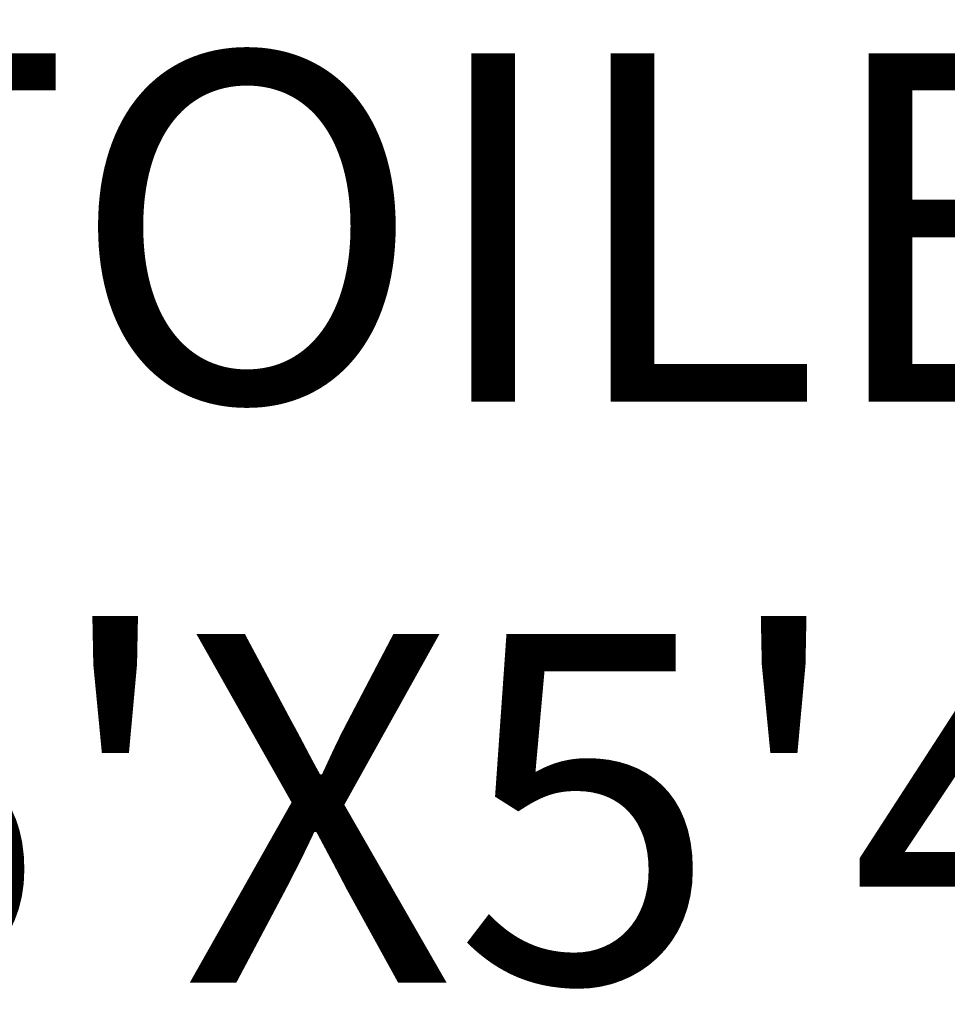
# Model space of a CAD drawing. Units: inches. Extents: x 2696 to 3240, y 1564 to 2310.
# Tile 73 of 76: x 3144 to 3168, y 2086 to 2111. Entities that reach past the tile are written whole.
import ezdxf

# ---------------------------------------------------------------- set-up
doc = ezdxf.new("R2010")
doc.units = ezdxf.units.IN
doc.layers.add('A-ANNO-DIMS', color=3, linetype='Continuous', lineweight=18)
doc.layers.add('A-AREA-IDEN', color=7, linetype='Continuous', lineweight=18)
doc.styles.add('TIMES NEW', font='times.ttf')
doc.styles.add('YQ_DIM', font='SUPEROS.SHX', dxfattribs={"width": 0.8, "bigfont": 'HZDX.SHX'})
doc.dimstyles.new('Siddhuu', dxfattribs={"dimtxt": 6, "dimasz": 2.5, "dimexe": 1.25, "dimexo": 0.625, "dimtad": 1, "dimdec": 1, "dimlunit": 4, "dimtxsty": 'TIMES NEW', "dimcen": 2.5, "dimclrd": 256, "dimclre": 1, "dimclrt": 7, "dimadec": 0, "dimazin": 0, "dimtfac": 1, "dimtdec": 1, "dimtmove": 0, "dimatfit": 3, "dimfxl": 1, "dimtolj": 1, "dimlwd": -1, "dimarcsym": 0})

# ---------------------------------------------------------------- blocks, each defined once
blk = doc.blocks.new('*D54')
at = {"layer": 'A-ANNO-DIMS', "color": 1, "lineweight": -2, "transparency": 16777216}
for p, q in [((3124.611, 1893.826), (3124.611, 2298.451)), ((3136.611, 1893.826), (3136.611, 2298.451))]:
    blk.add_line(p, q, dxfattribs=at)
at = {"layer": 'A-ANNO-DIMS', "transparency": 16777216}
for p, q in [((3127.111, 2297.201), (3134.111, 2297.201)), ((3136.611, 2297.201), (3155.757, 2297.201))]:
    blk.add_line(p, q, dxfattribs=at)
for points in [[(3127.111, 2297.618), (3127.111, 2296.784), (3124.611, 2297.201)], [(3134.111, 2297.618), (3134.111, 2296.784), (3136.611, 2297.201)]]:
    blk.add_solid(points, dxfattribs=at)
at = {"layer": 'Defpoints', "color": 0, "transparency": 16777216}
for p in [(3136.611, 2297.201), (3124.611, 1893.201), (3136.611, 1893.201)]:
    blk.add_point(p, dxfattribs=at)
at = {"layer": 'A-ANNO-DIMS', "color": 7, "transparency": 16777216, "insert": (3147.434, 2300.878), "char_height": 6, "attachment_point": 5, "style": 'TIMES NEW'}
blk.add_mtext('\\A1;1\'-0"', dxfattribs=at)

msp = doc.modelspace()

# ---------------------------------------------------------------- texts
at = {"layer": 'A-AREA-IDEN', "insert": (3138.221, 2110.067), "char_height": 9, "attachment_point": 1, "style": 'YQ_DIM'}
msp.add_mtext_dynamic_manual_height_columns('TOILET\\P5\'X5\'4.5"', width=48.00324, gutter_width=12.5, heights=[0], dxfattribs=at)

# ---------------------------------------------------------------- dimensions: what is measured, and where the dimension line sits
at = {"layer": 'A-ANNO-DIMS'}
dim = msp.add_linear_dim(base=(3136.611, 2297.201), p1=(3124.611, 1893.201), p2=(3136.611, 1893.201), dimstyle='Siddhuu', override={"dimdec": 1, "dimlfac": 1, "dimrnd": 0, "dimzin": 1, "dimdsep": 46, "dimlunit": 4, "dimfrac": 2}, dxfattribs=at)
dim.commit()
dim.dimension.update_dxf_attribs({"geometry": '*D54', "text_midpoint": (3147.434, 2300.878)})

doc.saveas('drawing.dxf')
